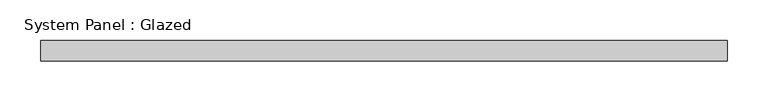
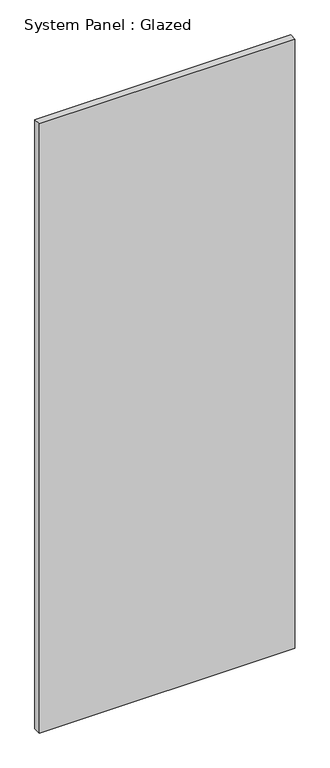
"""IFC4 building model written with IfcOpenShell, lengths in millimetres: plate geometry, System Panel : Glazed."""

from ifc_helpers import new_model, si_unit, origin, origin_with_axes, place, context, project, spatial, polyline, outline, extrude, source, transform, mapped, element, save


def system_panel_glazed_dbec328f(model_context):
    return source(origin(), model_context, "Body", "SweptSolid", [
        extrude(outline(polyline([(422.275, 19.05), (-422.275, 19.05), (-422.275, 44.45), (422.275, 44.45), (422.275, 19.05)])), origin_with_axes(), (0.0, 0.0, 1.0), 2127.3645985),
    ])


if __name__ == "__main__":
    model = new_model("IFC4")
    model_context = context("Model", 3, world=origin())
    ifc_project = project(units=[si_unit("LENGTHUNIT", "METRE", prefix="MILLI")], contexts=[model_context])
    site = spatial("IfcSite", under=ifc_project)
    building = spatial("IfcBuilding", under=site)
    placement = place(None, origin())
    system_panel_glazed_shape = system_panel_glazed_dbec328f(model_context)
    element("IfcPlate", 1, ObjectType="System Panel : Glazed", at=placement, inside=building, context=model_context, shape_type="MappedRepresentation", body=[
        mapped(system_panel_glazed_shape, transform((0.0, 0.0, 0.0), x_axis=(1.0, 0.0, 0.0), y_axis=(0.0, 1.0, 0.0), z_axis=(0.0, 0.0, 1.0))),
    ])
    save(model, "model.ifc")

# Revit data of these elements
# Type "System Panel : Glazed"
#   Construction Type Id = "GSP4R"
#   Analytic Construction = "1/8 in Pilkington single glazing"
#   Visual Light Transmittance = 0.9
#   Solar Heat Gain Coefficient = 0.86
#   Heat Transfer Coefficient (U) = 1.18115 BTU/(h·ft²·°F)
#   Define Thermal Properties by = 1
# Element 1 (IfcPlate, "System Panel : Glazed")
#   Materials on its faces: "Glass"
# Materials
#   "Glass": class "Glass", colour RGB 0 128 192, transparency 0.75, Description = "Soda Lime Glass", Cost = 0
